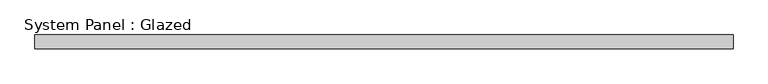
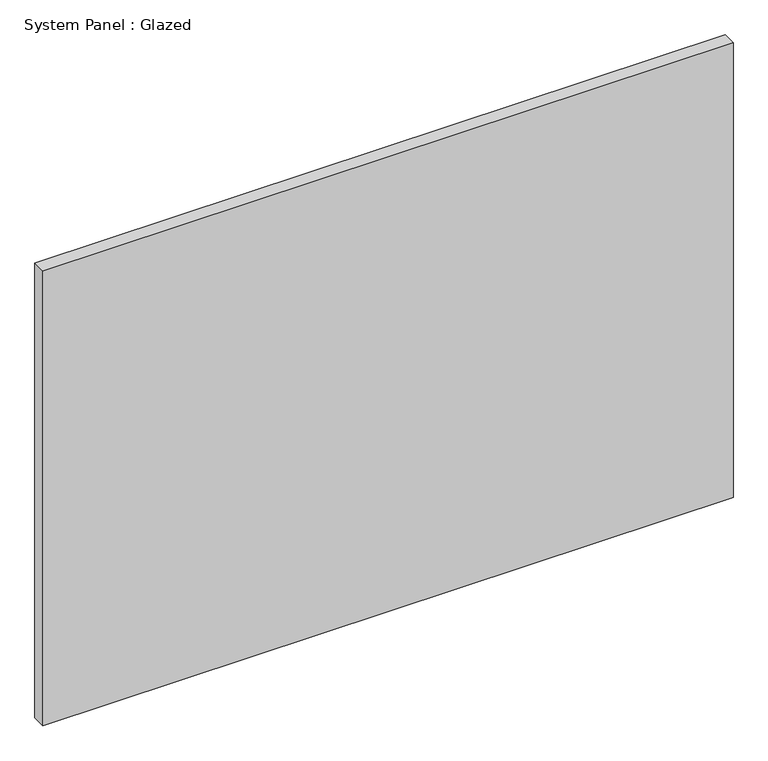
"""IFC4 building model written with IfcOpenShell, lengths in millimetres: plate geometry, System Panel : Glazed."""

from ifc_helpers import new_model, si_unit, origin, origin_with_axes, place, context, project, spatial, polyline, outline, extrude, source, transform, mapped, element, save


def system_panel_glazed_688ed8e9(model_context):
    return source(origin(), model_context, "Body", "SweptSolid", [
        extrude(outline(polyline([(634.947966, 19.05), (-634.947966, 19.05), (-634.947966, 44.45), (634.947966, 44.45), (634.947966, 19.05)])), origin_with_axes(), (0.0, 0.0, 1.0), 884.8113392),
    ])


if __name__ == "__main__":
    model = new_model("IFC4")
    model_context = context("Model", 3, world=origin())
    ifc_project = project(units=[si_unit("LENGTHUNIT", "METRE", prefix="MILLI")], contexts=[model_context])
    site = spatial("IfcSite", under=ifc_project)
    building = spatial("IfcBuilding", under=site)
    placement = place(None, origin())
    system_panel_glazed_shape = system_panel_glazed_688ed8e9(model_context)
    element("IfcPlate", 1, ObjectType="System Panel : Glazed", at=placement, inside=building, context=model_context, shape_type="MappedRepresentation", body=[
        mapped(system_panel_glazed_shape, transform((0.0, 0.0, 0.0), x_axis=(1.0, 0.0, 0.0), y_axis=(0.0, 1.0, 0.0), z_axis=(0.0, 0.0, 1.0))),
    ])
    save(model, "model.ifc")

# Revit data of these elements
# Type "System Panel : Glazed"
#   Construction Type Id = "GSP4R"
#   Analytic Construction = "1/8 in Pilkington single glazing"
#   Visual Light Transmittance = 0.9
#   Solar Heat Gain Coefficient = 0.86
#   Heat Transfer Coefficient (U) = 1.18115 BTU/(h·ft²·°F)
#   Define Thermal Properties by = 1
# Element 1 (IfcPlate, "System Panel : Glazed")
#   Materials on its faces: "Glass"
# Materials
#   "Glass": class "Glass", colour RGB 0 128 192, transparency 0.75, Description = "Soda Lime Glass", Cost = 0
